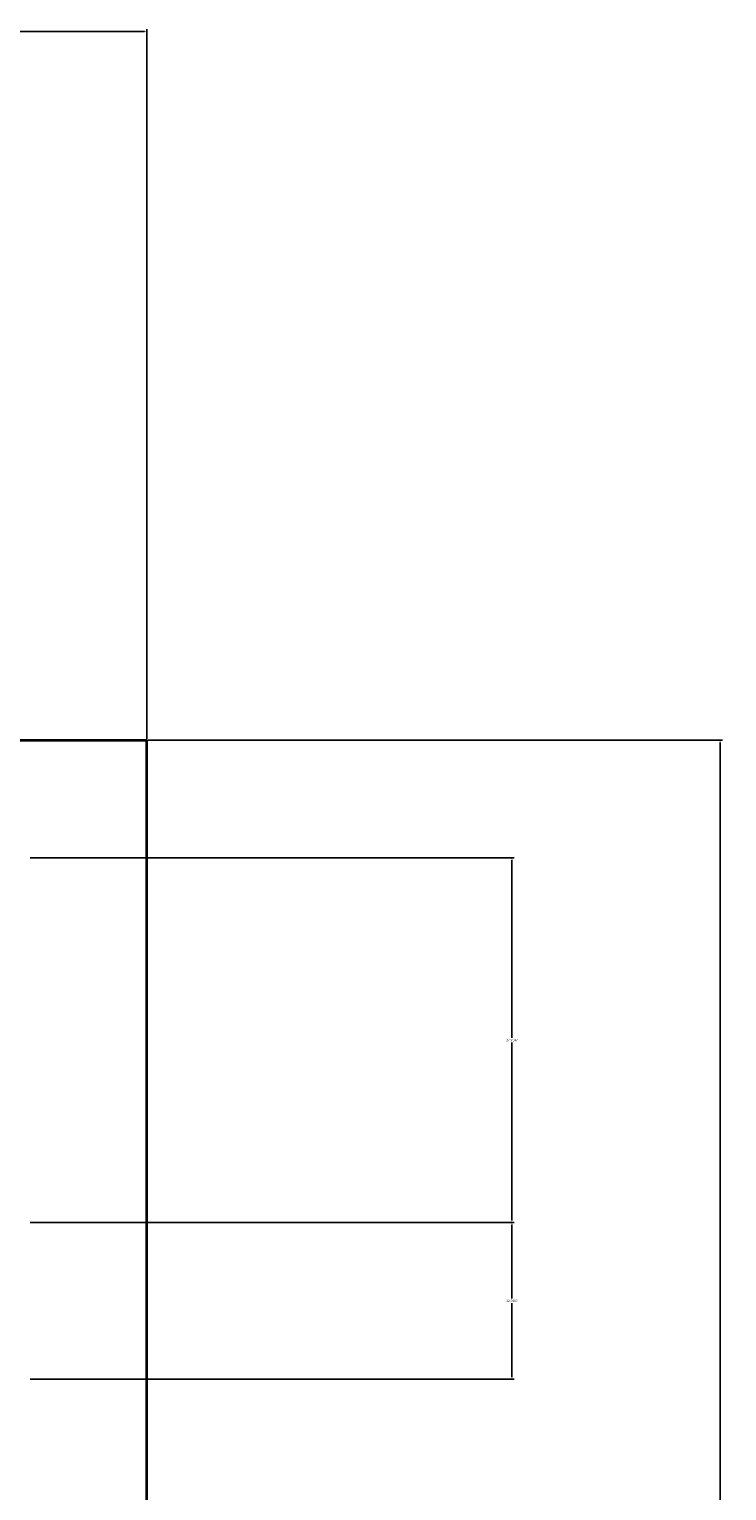
# Model space of a CAD drawing. Units: inches. Extents: x -26 to 788, y -42 to 505.
# Tile 8 of 9: x 298 to 352, y 374 to 486. Entities that reach past the tile are written whole.
import ezdxf

# ---------------------------------------------------------------- set-up
doc = ezdxf.new("R2010")
doc.units = ezdxf.units.IN
doc.header["$MEASUREMENT"] = 0
doc.layers.add('A-ANNO-DIMS', color=2, linetype='Continuous', lineweight=18)
doc.layers.add('A-WALL', color=7, linetype='Continuous', lineweight=35)
doc.styles.get("Standard").update_dxf_attribs({"font": 'arial.ttf'})
doc.dimstyles.get("Standard").update_dxf_attribs({"dimtxt": 0.18, "dimasz": 0.18, "dimexe": 0.18, "dimexo": 0.0625, "dimgap": 0.09, "dimtad": 0, "dimtih": 1, "dimtoh": 1, "dimdec": 4, "dimzin": 0, "dimdsep": 46, "dimtxsty": 'Standard', "dimcen": 0.09, "dimadec": 0, "dimazin": 0, "dimtfac": 1, "dimtdec": 4, "dimtofl": 0, "dimtmove": 0, "dimatfit": 3, "dimfxl": 1, "dimtolj": 1, "dimtzin": 0, "dimarcsym": 0})

# ---------------------------------------------------------------- blocks, each defined once
blk = doc.blocks.new('*D7')
at = {"layer": 'A-ANNO-DIMS', "color": 0, "lineweight": -2, "transparency": 16777216}
for p, q in [((2.95, 431.18), (2.95, 485.53)), ((307.45, 431.18), (307.45, 485.53)), ((3.13, 485.35), (154.6, 485.35)), ((307.27, 485.35), (155.81, 485.35))]:
    blk.add_line(p, q, dxfattribs=at)
at = {"layer": 'A-ANNO-DIMS', "color": 0, "transparency": 16777216}
for points in [[(3.13, 485.38), (3.13, 485.32), (2.95, 485.35)], [(307.27, 485.38), (307.27, 485.32), (307.45, 485.35)]]:
    blk.add_solid(points, dxfattribs=at)
at = {"layer": 'Defpoints', "color": 0, "transparency": 16777216}
for p in [(307.45, 485.35), (2.95, 431.12), (307.45, 431.12)]:
    blk.add_point(p, dxfattribs=at)
at = {"layer": 'A-ANNO-DIMS', "color": 0, "transparency": 16777216, "insert": (155.2, 485.35), "char_height": 0.18, "attachment_point": 5}
blk.add_mtext('\\A1;304.5000', dxfattribs=at)
blk = doc.blocks.new('*D8')
at = {"layer": 'A-ANNO-DIMS', "color": 0, "lineweight": -2, "transparency": 16777216}
for p, q in [((307.52, 431.12), (351.51, 431.12)), ((351.33, 430.94), (351.33, 216.8)), ((351.33, 2.3), (351.33, 216.44)), ((307.52, 2.12), (351.51, 2.12))]:
    blk.add_line(p, q, dxfattribs=at)
at = {"layer": 'A-ANNO-DIMS', "color": 0, "transparency": 16777216}
for points in [[(351.3, 430.94), (351.36, 430.94), (351.33, 431.12)], [(351.3, 2.3), (351.36, 2.3), (351.33, 2.12)]]:
    blk.add_solid(points, dxfattribs=at)
at = {"layer": 'Defpoints', "color": 0, "transparency": 16777216}
for p in [(307.45, 431.12), (307.45, 2.12), (351.33, 2.12)]:
    blk.add_point(p, dxfattribs=at)
at = {"layer": 'A-ANNO-DIMS', "color": 0, "transparency": 16777216, "insert": (351.33, 216.62), "char_height": 0.18, "attachment_point": 5}
blk.add_mtext('\\A1;429.0000', dxfattribs=at)
blk = doc.blocks.new('*D62')
at = {"layer": 'A-ANNO-DIMS', "color": 0, "lineweight": -2, "transparency": 16777216}
for p, q in [((298.52, 422.12), (335.58, 422.12)), ((335.4, 421.94), (335.4, 408.34)), ((335.4, 394.38), (335.4, 407.98)), ((298.52, 394.2), (335.58, 394.2))]:
    blk.add_line(p, q, dxfattribs=at)
at = {"layer": 'A-ANNO-DIMS', "color": 0, "transparency": 16777216}
for points in [[(335.37, 421.94), (335.43, 421.94), (335.4, 422.12)], [(335.37, 394.38), (335.43, 394.38), (335.4, 394.2)]]:
    blk.add_solid(points, dxfattribs=at)
at = {"layer": 'Defpoints', "color": 0, "transparency": 16777216}
for p in [(298.45, 422.12), (298.45, 394.2), (335.4, 394.2)]:
    blk.add_point(p, dxfattribs=at)
at = {"layer": 'A-ANNO-DIMS', "color": 0, "transparency": 16777216, "insert": (335.4, 408.16), "char_height": 0.18, "attachment_point": 5}
blk.add_mtext('\\A1;27.9147', dxfattribs=at)
blk = doc.blocks.new('*D63')
at = {"layer": 'A-ANNO-DIMS', "color": 0, "lineweight": -2, "transparency": 16777216}
for p, q in [((298.52, 394.2), (335.58, 394.2)), ((335.4, 394.02), (335.4, 388.38)), ((335.4, 382.38), (335.4, 388.02)), ((298.52, 382.2), (335.58, 382.2))]:
    blk.add_line(p, q, dxfattribs=at)
at = {"layer": 'A-ANNO-DIMS', "color": 0, "transparency": 16777216}
for points in [[(335.37, 394.02), (335.43, 394.02), (335.4, 394.2)], [(335.37, 382.38), (335.43, 382.38), (335.4, 382.2)]]:
    blk.add_solid(points, dxfattribs=at)
at = {"layer": 'Defpoints', "color": 0, "transparency": 16777216}
for p in [(298.45, 394.2), (298.45, 382.2), (335.4, 382.2)]:
    blk.add_point(p, dxfattribs=at)
at = {"layer": 'A-ANNO-DIMS', "color": 0, "transparency": 16777216, "insert": (335.4, 388.2), "char_height": 0.18, "attachment_point": 5}
blk.add_mtext('\\A1;12.0000', dxfattribs=at)

msp = doc.modelspace()

# ---------------------------------------------------------------- linework, layer by layer
at = {"layer": 'A-WALL'}
for p in [(2.95497, 431.11777), (307.45497, 308.37421)]:
    msp.add_line(p, (307.45497, 431.11777), dxfattribs=at)

# ---------------------------------------------------------------- dimensions: what is measured, and where the dimension line sits
at = {"layer": 'A-ANNO-DIMS'}
dim = msp.add_linear_dim(base=(307.45497, 485.35153), p1=(2.95497, 431.11777), p2=(307.45497, 431.11777), dimstyle='Standard', override={"dimclrd": 0, "dimclre": 0, "dimclrt": 0}, dxfattribs=at)
dim.commit()
dim.dimension.update_dxf_attribs({"geometry": '*D7', "text_midpoint": (155.20497, 485.35153)})
for base, p1, p2, override, picture, middle in [((351.33135, 2.11777), (307.45497, 431.11777), (307.45497, 2.11777), {"dimclrd": 0, "dimclre": 0, "dimclrt": 0}, '*D8', (351.33135, 216.61777)), ((335.40497, 394.20306), (298.45497, 422.11777), (298.45497, 394.20306), {"dimdec": 4, "dimlfac": 1, "dimrnd": 0, "dimzin": 0, "dimdsep": 46, "dimlunit": 2}, '*D62', (335.40497, 408.16041)), ((335.40497, 382.20306), (298.45497, 394.20306), (298.45497, 382.20306), {"dimdec": 4, "dimlfac": 1, "dimrnd": 0, "dimzin": 0, "dimdsep": 46, "dimlunit": 2}, '*D63', (335.40497, 388.20306))]:
    dim = msp.add_linear_dim(base=base, p1=p1, p2=p2, angle=90, dimstyle='Standard', override=override, dxfattribs=at)
    dim.commit()
    dim.dimension.update_dxf_attribs({"geometry": picture, "text_midpoint": middle})

doc.saveas('drawing.dxf')
